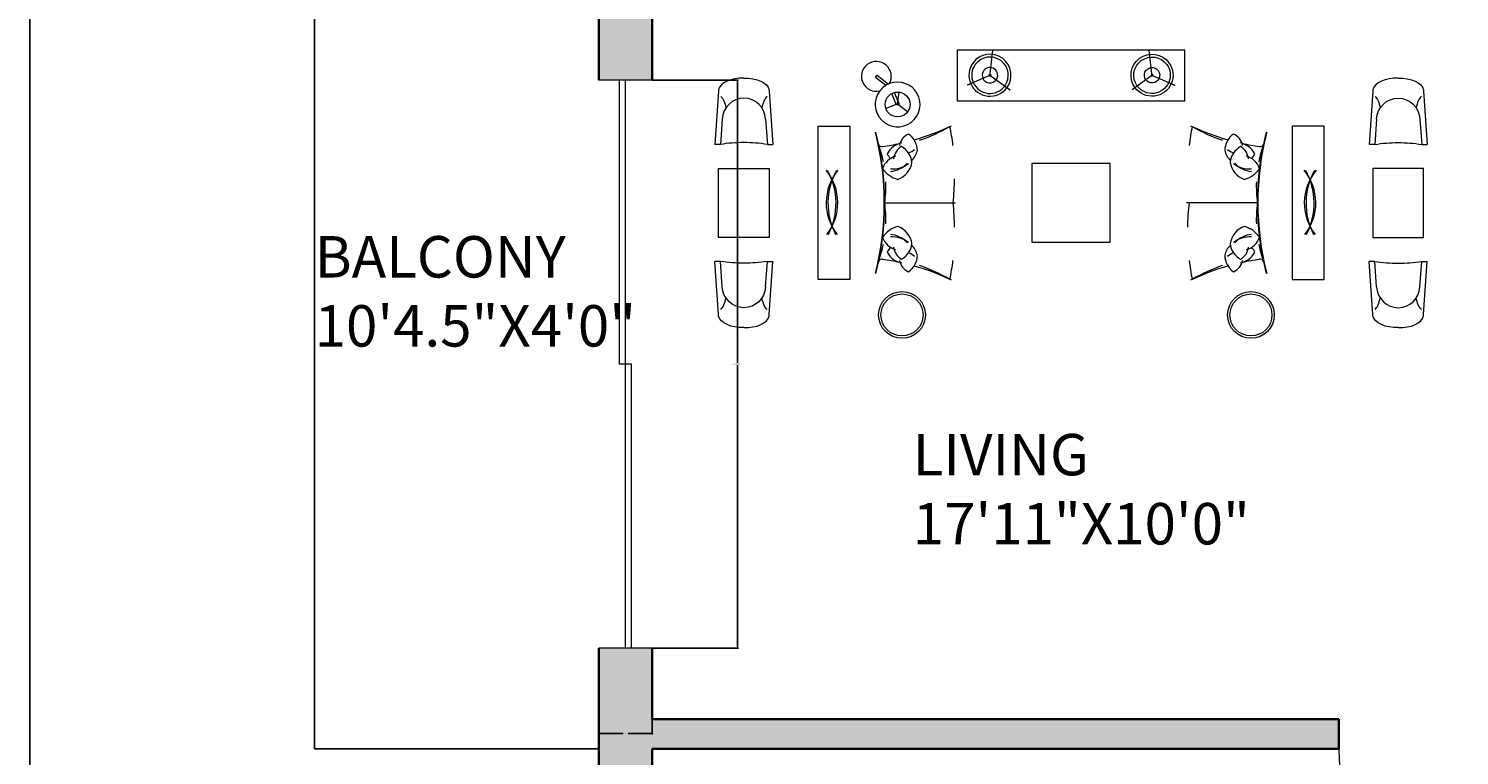
# Model space of a CAD drawing. Units: inches. Extents: x 2540 to 3167, y 3083 to 4007.
# Tile 10 of 15: x 2540 to 2782, y 3669 to 3791. Entities that reach past the tile are written whole.
import ezdxf

# ---------------------------------------------------------------- set-up
doc = ezdxf.new("R2010")
doc.units = ezdxf.units.IN
doc.set_wipeout_variables(frame=1)
for name, color, linetype, lineweight in [('A-ANNO-DIMS', 2, 'Continuous', 18), ('A-AREA-IDEN', 7, 'Continuous', 18), ('A-DOOR', 4, 'Continuous', 18), ('A-FLOR-EDGE', 7, 'Continuous', 25), ('A-FURN', 8, 'Continuous', 13)]:
    doc.layers.add(name, color=color, linetype=linetype, lineweight=lineweight)
doc.layers.add('A-WALL', color=143, linetype='Continuous', lineweight=35, true_color=0x7aafdf)
doc.layers.add('A-WALL-PATT', color=143, linetype='Continuous', lineweight=13, true_color=0x7aafdf)
doc.styles.get("Standard").update_dxf_attribs({"font": 'arial.ttf'})
doc.dimstyles.get("Standard").update_dxf_attribs({"dimtxt": 0.18, "dimasz": 0.18, "dimexe": 0.18, "dimexo": 0.0625, "dimgap": 0.09, "dimtad": 0, "dimtih": 1, "dimtoh": 1, "dimdec": 4, "dimzin": 0, "dimdsep": 46, "dimtxsty": 'Standard', "dimcen": 0.09, "dimadec": 0, "dimazin": 0, "dimtfac": 1, "dimtdec": 4, "dimtofl": 0, "dimtmove": 0, "dimatfit": 3, "dimfxl": 1, "dimtolj": 1, "dimtzin": 0, "dimarcsym": 0})

# ---------------------------------------------------------------- blocks, each defined once
blk = doc.blocks.new('A$C5805318C')
at = {"linetype": 'ByBlock'}
for p, q in [((1718, 2794), (1735, 2817)), ((1718, 2794), (1735, 2817)), ((1829, 2708), (1718, 2794)), ((1829, 2708), (1718, 2794)), ((1735, 2817), (1857, 2723)), ((1735, 2817), (1857, 2723)), ((1945, 2497), (1893, 2622)), ((1945, 2497), (1893, 2622)), ((1919, 2633), (1971, 2508)), ((1919, 2633), (1971, 2508)), ((1955, 2509), (1973, 2636)), ((1955, 2509), (1973, 2636)), ((1955, 2509), (1831, 2459)), ((1955, 2509), (1831, 2459)), ((1971, 2508), (1945, 2497)), ((1971, 2508), (1945, 2497)), ((1955, 2509), (2060, 2427)), ((1955, 2509), (2060, 2427))]:
    blk.add_line(p, q, dxfattribs=at)
for p, q in [((38, 2645), (0, 2075)), ((582, 2645), (620, 2075)), ((7041, 2645), (7003, 2075)), ((7585, 2645), (7623, 2075)), ((77, 2348), (59, 2075)), ((543, 2348), (561, 2075)), ((7080, 2348), (7062, 2075)), ((7545, 2348), (7564, 2075)), ((59, 2075), (0, 2075)), ((561, 2075), (620, 2075)), ((7062, 2075), (7003, 2075)), ((7564, 2075), (7623, 2075)), ((59, 824), (0, 824)), ((38, 254), (0, 824)), ((77, 551), (59, 824)), ((543, 551), (561, 824)), ((561, 824), (620, 824)), ((582, 254), (620, 824)), ((7062, 824), (7003, 824)), ((7041, 254), (7003, 824)), ((7080, 551), (7062, 824)), ((7545, 551), (7564, 824)), ((7564, 824), (7623, 824)), ((7585, 254), (7623, 824))]:
    blk.add_line(p, q)
for centre, radius in [((2002, 250), 250), ((2002, 250), 225), ((5737, 250), 250), ((5737, 250), 225)]:
    blk.add_circle(centre, radius)
for centre, radius, start, end in [((1727, 2805), 160, 331.0509, 282.9948), ((1955, 2504), 240, 111.272, 142.7738), ((1955, 2504), 240, 111.272, 142.7738)]:
    blk.add_arc(centre, radius, start, end, dxfattribs=at)
for points in [[(310, 2784), (175, 2792), (54, 2736), (40, 2660), (39, 2654), (38, 2649), (38, 2643)], [(310, 2784), (445, 2792), (566, 2736), (580, 2660), (581, 2654), (582, 2649), (582, 2643)], [(7313, 2784), (7178, 2792), (7057, 2736), (7042, 2660), (7041, 2654), (7041, 2649), (7041, 2643)], [(7313, 2784), (7448, 2792), (7569, 2736), (7583, 2660), (7584, 2654), (7585, 2649), (7585, 2643)], [(310, 116), (175, 108), (54, 163), (40, 240), (39, 245), (38, 251), (38, 256)], [(310, 116), (445, 108), (566, 163), (580, 240), (581, 245), (582, 251), (582, 256)], [(7313, 116), (7178, 108), (7057, 163), (7042, 240), (7041, 245), (7041, 251), (7041, 256)], [(7313, 116), (7448, 108), (7569, 163), (7583, 240), (7584, 245), (7585, 251), (7585, 256)]]:
    blk.add_open_spline(points, degree=3, knots=[0, 0, 0, 0, 1, 1, 1, 2, 2, 2, 2])
for points in [[(62, 2590), (86, 2572), (108, 2522), (117, 2466)], [(310, 2572), (188, 2572), (86, 2474), (77, 2348)], [(543, 2348), (534, 2474), (433, 2572), (310, 2572)], [(558, 2590), (535, 2572), (512, 2522), (503, 2466)], [(7065, 2590), (7088, 2572), (7110, 2522), (7119, 2466)], [(7080, 2348), (7089, 2474), (7190, 2572), (7313, 2572)], [(7313, 2572), (7435, 2572), (7537, 2474), (7545, 2348)], [(7561, 2590), (7537, 2572), (7515, 2522), (7506, 2466)], [(310, 2096), (226, 2096), (142, 2089), (59, 2075)], [(561, 2075), (478, 2089), (394, 2096), (310, 2096)], [(7062, 2075), (7145, 2089), (7229, 2096), (7313, 2096)], [(7313, 2096), (7397, 2096), (7481, 2089), (7564, 2075)], [(310, 804), (226, 804), (142, 810), (59, 824)], [(561, 824), (478, 810), (394, 804), (310, 804)], [(7062, 824), (7145, 810), (7229, 804), (7313, 804)], [(7313, 804), (7397, 804), (7481, 810), (7564, 824)], [(310, 328), (188, 328), (86, 425), (77, 551)], [(543, 551), (534, 425), (433, 328), (310, 328)], [(7080, 551), (7089, 425), (7190, 328), (7313, 328)], [(7313, 328), (7435, 328), (7537, 425), (7545, 551)], [(62, 310), (86, 327), (108, 378), (117, 434)], [(558, 310), (535, 327), (512, 378), (503, 434)], [(7065, 310), (7088, 327), (7110, 378), (7119, 434)], [(7561, 310), (7537, 327), (7515, 378), (7506, 434)]]:
    blk.add_open_spline(points, degree=3)
for points in [[(2561, 3114), (2561, 2514), (5061, 2514), (5061, 3114)], [(1474, 600), (1074, 600), (1074, 2300), (1474, 2300)], [(2575, 1450), (2574, 1519), (2572, 1654), (2567, 1805), (2559, 1944), (2549, 2088), (2540, 2188), (2531, 2276), (2527, 2314), (1674, 2200), (1674, 1450), (1674, 699), (2527, 585), (2531, 623), (2540, 712), (2549, 811), (2559, 956), (2567, 1094), (2572, 1246), (2574, 1380)], [(5048, 1450), (5048, 1519), (5051, 1654), (5056, 1805), (5064, 1944), (5074, 2088), (5083, 2188), (5091, 2276), (5096, 2314), (5949, 2200), (5949, 1450), (5949, 699), (5096, 585), (5091, 623), (5083, 712), (5074, 811), (5064, 956), (5056, 1094), (5051, 1246), (5048, 1380)], [(6149, 600), (6549, 600), (6549, 2300), (6149, 2300)], [(610, 1050), (10, 1050), (10, 1850), (610, 1850)], [(3361, 1000), (4261, 1000), (4261, 1900), (3361, 1900)], [(7013, 1050), (7613, 1050), (7613, 1850), (7013, 1850)]]:
    blk.add_wipeout(points, dxfattribs=at)
for p, q in [((2943, 2802), (2974, 3081)), ((2968, 3032), (2974, 3078)), ((4680, 2802), (4649, 3081)), ((4654, 3032), (4649, 3078)), ((2958, 2823), (2701, 2710)), ((2932, 2826), (3159, 2659)), ((4690, 2826), (4464, 2659)), ((4665, 2823), (4922, 2710)), ((2746, 2730), (2704, 2712)), ((3119, 2688), (3156, 2661)), ((4504, 2688), (4467, 2661)), ((4877, 2730), (4919, 2712))]:
    blk.add_line(p, q, dxfattribs=at)
for p, q in [((1817, 1450), (2575, 1450)), ((5805, 1450), (5048, 1450))]:
    blk.add_line(p, q)
for points in [[(2591, 3084), (2591, 2544), (5031, 2544), (5031, 3084)], [(1444, 630), (1104, 630), (1104, 2270), (1444, 2270)], [(6179, 630), (6519, 630), (6519, 2270), (6179, 2270)], [(3391, 1030), (4231, 1030), (4231, 1870), (3391, 1870)], [(580, 1080), (40, 1080), (40, 1820), (580, 1820)], [(7043, 1080), (7583, 1080), (7583, 1820), (7043, 1820)]]:
    blk.add_lwpolyline(points, close=True, dxfattribs=at)
blk.add_circle((1955, 2504), 133, dxfattribs=at)
blk.add_circle((1955, 2504), 133, dxfattribs=at)
for centre, radius, start, end in [((1955, 2504), 240, 142.7738, 111.272), ((-1206, 1450), 3024, 345.5057, 14.4943), ((2141, 2032), 169, 113.788, 168.6748), ((1945, 2005), 222, 1.4651, 55.0097), ((1435, 4574), 2546, 285.8776, 295.5087), ((6188, 4574), 2546, 244.4913, 254.1224), ((5678, 2005), 222, 124.9903, 178.5349), ((5482, 2032), 169, 11.3252, 66.212), ((8829, 1450), 3024, 165.5057, 194.4943), ((1785, 2087), 34.6, 193.5328, 287.2771), ((1435, 4574), 2546, 278.134, 282.3755), ((2038, 1878), 217, 100.5196, 152.9581), ((2081, 1906), 169, 119.788, 174.6748), ((1889, 1858), 222, 7.4651, 61.0097), ((1947, 2064), 226, 314.9669, 346.4215), ((5676, 2064), 226, 193.5785, 225.0331), ((5734, 1858), 222, 118.9903, 172.5349), ((5585, 1878), 217, 27.0419, 79.4804), ((5542, 1906), 169, 5.3252, 60.212), ((6188, 4574), 2546, 257.6245, 261.866), ((5838, 2087), 34.6, 252.7229, 346.4672), ((1996, 1742), 217, 106.5196, 158.9581), ((2095, 2106), 282, 207.4684, 220.0792), ((1885, 1917), 226, 288.0023, 352.4215), ((5738, 1917), 226, 187.5785, 251.9977), ((5627, 1742), 217, 21.0419, 73.4804), ((5528, 2106), 282, 319.9208, 332.5316), ((769, 1450), 546, 321.7197, 39.6872), ((1737, 1450), 546, 140.3128, 218.2803), ((564, 1447), 732, 332.7542, 28.6527), ((1942, 1447), 732, 151.3473, 207.2458), ((2028, 1975), 282, 213.4684, 255.3384), ((5595, 1975), 282, 284.6616, 326.5316), ((5885, 1450), 546, 321.7197, 39.6872), ((6854, 1450), 546, 140.3128, 218.2803), ((5681, 1447), 732, 332.7542, 28.6527), ((7058, 1447), 732, 151.3473, 207.2458), ((2028, 924), 282, 104.6616, 146.5316), ((1996, 1158), 217, 201.0419, 253.4804), ((1885, 982), 226, 7.5785, 71.9977), ((5738, 982), 226, 108.0023, 172.4215), ((5595, 924), 282, 33.4684, 75.3384), ((5627, 1158), 217, 286.5196, 338.9581), ((2095, 793), 282, 139.9208, 152.5316), ((2038, 1021), 217, 207.0419, 259.4804), ((2081, 993), 169, 185.3252, 240.212), ((1889, 1041), 222, 298.9903, 352.5349), ((1947, 836), 226, 13.5785, 45.0331), ((5676, 836), 226, 134.9669, 166.4215), ((5734, 1041), 222, 187.4651, 241.0097), ((5585, 1021), 217, 280.5196, 332.9581), ((5542, 993), 169, 299.788, 354.6748), ((5528, 793), 282, 27.4684, 40.0792), ((1785, 813), 34.6, 72.7229, 166.4672), ((1435, -1675), 2546, 77.6245, 81.866), ((2141, 867), 169, 191.3252, 246.212), ((1945, 894), 222, 304.9903, 358.5349), ((1435, -1675), 2546, 64.4913, 74.1224), ((6188, -1675), 2546, 105.8776, 115.5087), ((5678, 894), 222, 181.4651, 235.0097), ((5482, 867), 169, 293.788, 348.6748), ((6188, -1675), 2546, 98.134, 102.3755), ((5838, 813), 34.6, 13.5328, 107.2771)]:
    blk.add_arc(centre, radius, start, end, dxfattribs=at)
for centre, radius, start, end in [((-1206, 1450), 3019, 345.5057, 14.4943), ((1640, 3765), 1733, 288.4757, 300.3241), ((-91, 1753), 2657, 6.7363, 11.1857), ((7714, 1753), 2657, 168.8143, 173.2637), ((5982, 3765), 1733, 239.6759, 251.5243), ((8829, 1450), 3019, 165.5057, 194.4943), ((477, 1627), 1352, 11.274, 19.5243), ((1964, 2245), 282, 292.5627, 307.9208), ((5659, 2245), 282, 232.0792, 247.4373), ((7146, 1627), 1352, 160.4757, 168.726), ((1853, 2068), 282, 275.0195, 316.8895), ((1899, 2095), 282, 266.0508, 307.9208), ((5723, 2095), 282, 232.0792, 273.9492), ((5769, 2068), 282, 223.1105, 264.9805), ((-91, 1753), 2657, 353.4417, 359.0402), ((477, 1627), 1352, 352.4802, 2.0119), ((7146, 1627), 1352, 177.9881, 187.5198), ((477, 1273), 1352, 357.9881, 7.5198), ((-91, 1146), 2657, 0.9598, 6.5583), ((7714, 1146), 2657, 173.4417, 179.0402), ((7146, 1273), 1352, 172.4802, 182.0119), ((1853, 831), 282, 43.1105, 84.9805), ((1899, 804), 282, 52.0792, 93.9492), ((5723, 804), 282, 86.0508, 127.9208), ((5769, 831), 282, 95.0195, 136.8895), ((477, 1273), 1352, 340.4757, 348.726), ((7146, 1273), 1352, 191.274, 199.5243), ((1964, 654), 282, 52.0792, 67.4373), ((1640, -865), 1733, 59.6759, 71.5243), ((-91, 1146), 2657, 348.8143, 353.2637), ((7714, 1146), 2657, 186.7363, 191.1857), ((5982, -865), 1733, 108.4757, 120.3241), ((5659, 654), 282, 112.5627, 127.9208)]:
    blk.add_arc(centre, radius, start, end)
for major_axis, start_param, end_param in [((-159, 159), 3.292387, 6.433979), ((-159, 159), 0.150794, 3.292387), ((-138, 138), 0.150794, 3.292387), ((-138, 138), 3.292387, 6.433979), ((-58.4, 58.4), 0.150794, 3.292387), ((-58.4, 58.4), 3.292387, 6.433979)]:
    blk.add_ellipse((2944, 2817), major_axis=major_axis, ratio=1, start_param=start_param, end_param=end_param, dxfattribs=at)
at = {"linetype": 'ByBlock', "extrusion": (0, 0, -1)}
for major_axis, start_param, end_param in [((159, 159), 3.292387, 6.433979), ((138, 138), 3.292387, 6.433979), ((159, 159), 0.150794, 3.292387), ((138, 138), 0.150794, 3.292387), ((-58.4, 58.4), 4.863183, 8.004776), ((-58.4, 58.4), 1.72159, 4.863183)]:
    blk.add_ellipse((4678, 2817), major_axis=major_axis, ratio=1, start_param=start_param, end_param=end_param, dxfattribs=at)
blk = doc.blocks.new('DOOR-SWING-36IN')
for p, q in [((36, 0), (0, 0)), ((36, 1), (0.01, 1)), ((36, 1), (36, 0))]:
    blk.add_line(p, q)
blk.add_arc((36, 0), 36, 90, 180)
blk = doc.blocks.new('DOOR-SLIDING-96IN')
for p, q in [((9, 96), (0, 96)), ((3.5, 48), (3.5, 96)), ((4.5, 0), (4.5, 96)), ((5.5, 48), (3.5, 48)), ((5.5, 0), (5.5, 48)), ((9, 0), (0, 0))]:
    blk.add_line(p, q)
blk = doc.blocks.new('*D23')
at = {"layer": 'A-ANNO-DIMS', "color": 0, "lineweight": -2, "transparency": 16777216}
for p, q in [((2645.57, 3782.71), (2660.09, 3782.71)), ((2659.91, 3782.53), (2659.91, 3734.9)), ((2659.91, 3686.89), (2659.91, 3734.53)), ((2645.57, 3686.71), (2660.09, 3686.71))]:
    blk.add_line(p, q, dxfattribs=at)
at = {"layer": 'A-ANNO-DIMS', "color": 0, "transparency": 16777216}
for points in [[(2659.88, 3782.53), (2659.94, 3782.53), (2659.91, 3782.71)], [(2659.88, 3686.89), (2659.94, 3686.89), (2659.91, 3686.71)]]:
    blk.add_solid(points, dxfattribs=at)
at = {"layer": 'Defpoints', "color": 0, "transparency": 16777216}
for p in [(2645.51, 3782.71), (2659.91, 3782.71), (2645.51, 3686.71)]:
    blk.add_point(p, dxfattribs=at)
at = {"layer": 'A-ANNO-DIMS', "color": 0, "transparency": 16777216, "insert": (2659.91, 3734.71), "char_height": 0.18, "attachment_point": 5}
blk.add_mtext('\\A1;SLIDER 96 TYP.', dxfattribs=at)
blk = doc.blocks.new('*D24')
at = {"layer": 'A-ANNO-DIMS', "color": 0, "lineweight": -2, "transparency": 16777216}
for p, q in [((2636.51, 3686.65), (2636.51, 3672.13)), ((2645.51, 3686.65), (2645.51, 3672.13)), ((2636.69, 3672.31), (2640.55, 3672.31)), ((2645.33, 3672.31), (2641.47, 3672.31))]:
    blk.add_line(p, q, dxfattribs=at)
at = {"layer": 'A-ANNO-DIMS', "color": 0, "transparency": 16777216}
for points in [[(2636.69, 3672.34), (2636.69, 3672.28), (2636.51, 3672.31)], [(2645.33, 3672.34), (2645.33, 3672.28), (2645.51, 3672.31)]]:
    blk.add_solid(points, dxfattribs=at)
at = {"layer": 'Defpoints', "color": 0, "transparency": 16777216}
for p in [(2636.51, 3686.71), (2645.51, 3686.71), (2645.51, 3672.31)]:
    blk.add_point(p, dxfattribs=at)
at = {"layer": 'A-ANNO-DIMS', "color": 0, "transparency": 16777216, "insert": (2641.01, 3672.31), "char_height": 0.18, "attachment_point": 5}
blk.add_mtext('\\A1;9 TYP.', dxfattribs=at)
blk = doc.blocks.new('*D44')
at = {"layer": 'A-ANNO-DIMS', "color": 0, "lineweight": -2, "transparency": 16777216}
for p, q in [((2771.45, 3964.71), (2540.23, 3964.71)), ((2540.41, 3964.53), (2540.41, 3545.4)), ((2540.41, 3125.89), (2540.41, 3545.03)), ((2810.45, 3125.71), (2540.23, 3125.71))]:
    blk.add_line(p, q, dxfattribs=at)
at = {"layer": 'A-ANNO-DIMS', "color": 0, "transparency": 16777216}
for points in [[(2540.38, 3964.53), (2540.44, 3964.53), (2540.41, 3964.71)], [(2540.38, 3125.89), (2540.44, 3125.89), (2540.41, 3125.71)]]:
    blk.add_solid(points, dxfattribs=at)
at = {"layer": 'Defpoints', "color": 0, "transparency": 16777216}
for p in [(2540.41, 3964.71), (2771.51, 3964.71), (2810.51, 3125.71)]:
    blk.add_point(p, dxfattribs=at)
at = {"layer": 'A-ANNO-DIMS', "color": 0, "transparency": 16777216, "insert": (2540.41, 3545.21), "char_height": 0.18, "attachment_point": 5}
blk.add_mtext('\\A1;839', dxfattribs=at)

msp = doc.modelspace()

# ---------------------------------------------------------------- hatches: boundary and pattern name
at = {"layer": 'A-WALL-PATT'}
h = msp.add_hatch(color=256, dxfattribs=at)
h.dxf.hatch_style = 1
h.paths.add_polyline_path([(2805.51, 3803.71), (2800.51, 3803.71), (2800.51, 3799.71), (2621.51, 3799.71), (2621.51, 3823.71), (2612.51, 3823.71), (2612.51, 3794.71), (2636.51, 3794.71), (2636.51, 3782.71), (2645.51, 3782.71), (2645.51, 3794.71), (2805.51, 3794.71)])
h.paths.add_polyline_path([(2810.51, 3564.71), (2868.51, 3564.71), (2868.51, 3627.71), (2872.51, 3627.71), (2872.51, 3636.71), (2864.51, 3636.71), (2864.51, 3674.71), (2797.51, 3674.71), (2797.51, 3669.71), (2801.51, 3669.71), (2801.51, 3628.63), (2806.51, 3628.63), (2806.51, 3669.71), (2859.51, 3669.71), (2859.51, 3573.71), (2806.51, 3573.71), (2806.51, 3598.63), (2801.51, 3598.63), (2801.51, 3549.71), (2645.51, 3549.71), (2645.51, 3573.71), (2636.51, 3573.71), (2636.51, 3516.71), (2645.51, 3516.71), (2645.51, 3540.71), (2801.51, 3540.71), (2801.51, 3504.71), (2801.51, 3500.71), (2806.51, 3500.71), (2806.51, 3504.71), (2859.51, 3504.71), (2859.51, 3420.71), (2806.51, 3420.71), (2806.51, 3470.71), (2801.51, 3470.71), (2801.51, 3420.71), (2797.51, 3420.71), (2797.51, 3415.71), (2864.51, 3415.71), (2864.51, 3453.71), (2868.51, 3453.71), (2868.51, 3513.71), (2810.51, 3513.71)])
h.paths.add_polyline_path([(2645.51, 3415.71), (2761.51, 3415.71), (2761.51, 3420.71), (2645.51, 3420.71), (2645.51, 3444.71), (2636.51, 3444.71), (2636.51, 3403.71), (2645.51, 3403.71)])
h.paths.add_polyline_path([(2645.51, 3307.71), (2636.51, 3307.71), (2636.51, 3295.71), (2612.51, 3295.71), (2612.51, 3149.71), (2645.51, 3149.71), (2645.51, 3158.71), (2621.51, 3158.71), (2621.51, 3290.71), (2801.51, 3290.71), (2801.51, 3286.71), (2806.51, 3286.71), (2806.51, 3295.71), (2645.51, 3295.71)])
h.paths.add_polyline_path([(2762.01, 3158.71), (2746.51, 3158.71), (2746.51, 3240.71), (2750.51, 3240.71), (2750.51, 3245.71), (2741.51, 3245.71), (2741.51, 3158.71), (2717.51, 3158.71), (2717.51, 3149.71), (2762.01, 3149.71)], flags=17)
h.paths.add_polyline_path([(2810.51, 3173.71), (2822.51, 3173.71), (2822.51, 3182.71), (2806.51, 3182.71), (2806.51, 3250.71), (2801.51, 3250.71), (2801.51, 3245.71), (2780.51, 3245.71), (2780.51, 3240.71), (2801.51, 3240.71), (2801.51, 3158.71), (2786.01, 3158.71), (2786.01, 3149.71), (2810.51, 3149.71)])
h.paths.add_polyline_path([(2931.51, 3290.71), (2935.51, 3290.71), (2935.51, 3295.71), (2926.51, 3295.71), (2926.51, 3182.71), (2910.51, 3182.71), (2910.51, 3173.71), (2922.51, 3173.71), (2922.51, 3149.71), (2987.51, 3149.71), (2987.51, 3158.71), (2931.51, 3158.71)])
h.paths.add_polyline_path([(3124.51, 3295.71), (3086.51, 3295.71), (3018.51, 3295.71), (3018.51, 3290.71), (3115.51, 3290.71), (3115.51, 3158.71), (3059.51, 3158.71), (3059.51, 3149.71), (3124.51, 3149.71)])
h.paths.add_polyline_path([(2988.51, 3295.71), (2984.51, 3295.71), (2984.51, 3349.71), (3086.51, 3349.71), (3086.51, 3320.71), (3124.51, 3320.71), (3124.51, 3354.71), (3071.51, 3354.71), (3071.51, 3358.71), (3062.51, 3358.71), (3062.51, 3354.71), (2979.51, 3354.71), (2979.51, 3295.71), (2971.51, 3295.71), (2971.51, 3290.71), (2988.51, 3290.71)])
h.paths.add_polyline_path([(3095.51, 3325.71), (3095.51, 3349.71), (3119.51, 3349.71), (3119.51, 3325.71)], flags=16)
h.paths.add_polyline_path([(3124.51, 3462.71), (3071.51, 3462.71), (3071.51, 3627.71), (3124.51, 3627.71), (3124.51, 3693.71), (3095.51, 3693.71), (3095.51, 3702.71), (3086.51, 3702.71), (3086.51, 3684.71), (3086.51, 3636.71), (2930.51, 3636.71), (2930.51, 3768.71), (2934.51, 3768.71), (2934.51, 3773.71), (2930.51, 3773.71), (2925.51, 3773.71), (2925.51, 3730.71), (2864.51, 3730.71), (2864.51, 3760.71), (2859.51, 3760.71), (2859.51, 3725.71), (2925.51, 3725.71), (2925.51, 3636.71), (2908.51, 3636.71), (2908.51, 3627.71), (3062.51, 3627.71), (3062.51, 3543.71), (2930.51, 3543.71), (2930.51, 3534.71), (2993.51, 3534.71), (2993.51, 3516.71), (3002.51, 3516.71), (3002.51, 3534.71), (3062.51, 3534.71), (3062.51, 3462.71), (3002.51, 3462.71), (3002.51, 3480.71), (2993.51, 3480.71), (2993.51, 3462.71), (2916.51, 3462.71), (2916.51, 3453.71), (2926.51, 3453.71), (2926.51, 3361.71), (2859.51, 3361.71), (2859.51, 3338.71), (2864.51, 3338.71), (2864.51, 3356.71), (2926.51, 3356.71), (2926.51, 3338.71), (2931.51, 3338.71), (2931.51, 3453.71), (3062.51, 3453.71), (3062.51, 3448.21), (3071.51, 3448.21), (3071.51, 3453.71), (3124.51, 3453.71)])
h = msp.add_hatch(color=256, dxfattribs=at)
h.dxf.hatch_style = 1
h.paths.add_polyline_path([(3095.51, 3788.71), (3086.51, 3788.71), (3086.51, 3773.71), (3015.51, 3773.71), (3015.51, 3768.71), (3086.51, 3768.71), (3086.51, 3750.71), (3095.51, 3750.71)])
h.paths.add_polyline_path([(2645.51, 3669.71), (2761.51, 3669.71), (2761.51, 3674.71), (2645.51, 3674.71), (2645.51, 3686.71), (2636.51, 3686.71), (2636.51, 3645.71), (2645.51, 3645.71)])

# ---------------------------------------------------------------- linework, layer by layer
at = {"layer": 'A-FLOR-EDGE'}
for p, q in [((2588.51, 3805.11), (2588.51, 3669.71)), ((2588.51, 3669.71), (2636.51, 3669.71))]:
    msp.add_line(p, q, dxfattribs=at)
at = {"layer": 'A-WALL'}
for p, q in [((2636.51, 3794.71), (2636.51, 3782.71)), ((2645.51, 3794.71), (2645.51, 3782.71)), ((2636.51, 3686.71), (2636.51, 3403.71)), ((2645.51, 3686.71), (2645.51, 3674.71)), ((2645.51, 3674.71), (2761.51, 3674.71)), ((2761.51, 3674.71), (2761.51, 3669.71)), ((2645.51, 3669.71), (2645.51, 3549.71)), ((2645.51, 3669.71), (2761.51, 3669.71))]:
    msp.add_line(p, q, dxfattribs=at)

# ---------------------------------------------------------------- block references
at = {"layer": 'A-DOOR'}
msp.add_blockref('DOOR-SLIDING-96IN', (2636.51, 3686.71), dxfattribs=at)
at = {"layer": 'A-DOOR', "rotation": 89.99999999999872}
msp.add_blockref('DOOR-SWING-36IN', (2797.51, 3633.71), dxfattribs=at)

# ---------------------------------------------------------------- texts
at = {"layer": 'A-AREA-IDEN', "char_height": 7, "attachment_point": 1}
for s, width, insert in [('BALCONY\\P10\'4.5"X4\'0"', 97.3161, (2588.51, 3756.35)), ('LIVING \\P17\'11"X10\'0"', 34.8892, (2689.53, 3722.92))]:
    msp.add_mtext_dynamic_manual_height_columns(s, width=width, gutter_width=12.5, heights=[0], dxfattribs=dict(at, insert=insert))

# ---------------------------------------------------------------- dimensions: what is measured, and where the dimension line sits
at = {"layer": 'A-ANNO-DIMS'}
dim = msp.add_linear_dim(base=(2645.51, 3672.31), p1=(2636.51, 3686.71), p2=(2645.51, 3686.71), text='<> TYP.', dimstyle='Standard', override={"dimdec": 0, "dimlfac": 1, "dimrnd": 0, "dimzin": 0, "dimdsep": 46, "dimlunit": 2}, dxfattribs=at)
dim.commit()
dim.dimension.update_dxf_attribs({"geometry": '*D24', "text_midpoint": (2641.01, 3672.31)})

# ---------------------------------------------------------------- next in the draw order: block references
at = {"layer": 'A-FURN', "xscale": 0.0157806756092575, "yscale": 0.0157806756092575, "zscale": 0.0157806756092575}
msp.add_blockref('A$C5805318C', (2656.12, 3739.08), dxfattribs=at)

# ---------------------------------------------------------------- next in the draw order: dimensions: what is measured, and where the dimension line sits
at = {"layer": 'A-ANNO-DIMS'}
dim = msp.add_linear_dim(base=(2540.41, 3964.71), p1=(2810.51, 3125.71), p2=(2771.51, 3964.71), angle=90, dimstyle='Standard', override={"dimdec": 0, "dimlfac": 1, "dimrnd": 0, "dimzin": 0, "dimdsep": 46, "dimlunit": 2}, dxfattribs=at)
dim.commit()
dim.dimension.update_dxf_attribs({"geometry": '*D44', "text_midpoint": (2540.41, 3545.21)})
dim = msp.add_linear_dim(base=(2659.91, 3782.71), p1=(2645.51, 3686.71), p2=(2645.51, 3782.71), angle=90, text='SLIDER <> TYP.', dimstyle='Standard', override={"dimdec": 0, "dimlfac": 1, "dimrnd": 0, "dimzin": 0, "dimdsep": 46, "dimlunit": 2}, dxfattribs=at)
dim.commit()
dim.dimension.update_dxf_attribs({"geometry": '*D23', "text_midpoint": (2659.91, 3734.71)})

doc.saveas('drawing.dxf')
